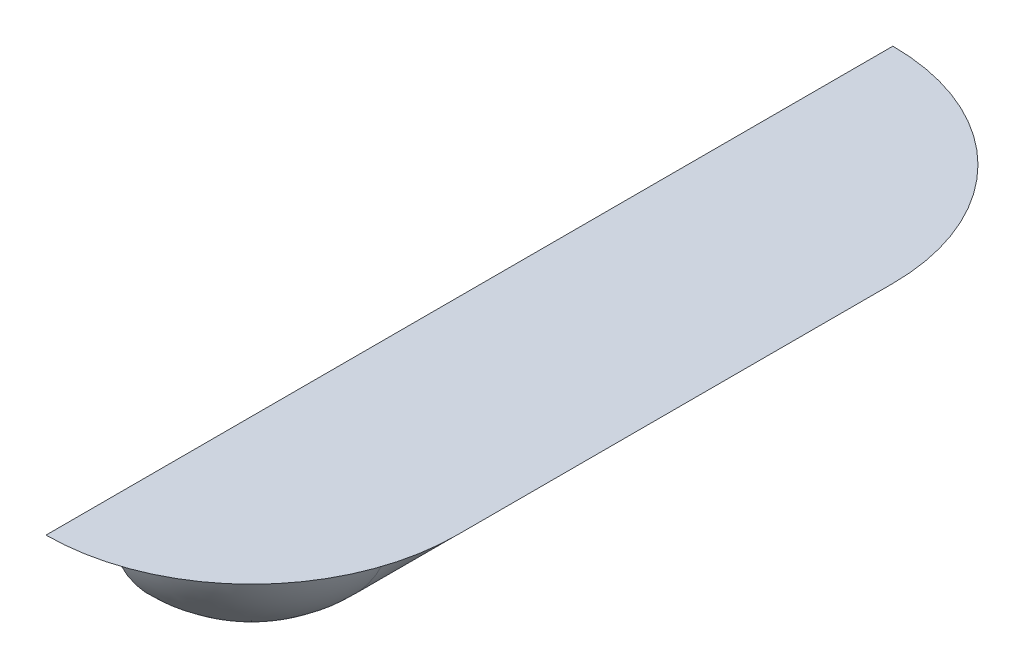
SolidWorks part; units mm, degrees
material "Plain Carbon Steel"
ref_plane "Plane1" through (0, 0, 0) normal (0, 0, 1) x (1, 0, 0)
ref_plane "Plane2" through (0, 0, 0) normal (0, 1, 0) x (1, 0, 0)
ref_plane "Plane3" through (0, 0, 0) normal (1, 0, 0) x (0, 0, -1)
sketch "Base Profile Sketch" plane through (0, 0, 0) normal (0, 0, 1) x (1, 0, 0)
  line L0 (-25, 0) -> (25, 0)
  line L1 (-25, 0) -> (-25, 3.4642)
  line L2 (25, 3.4642) -> (-25, 3.4642)
  line L3 (25, 3.4642) -> (25, 0)
  line L4 (0, 0) -> (0, 3.4642) construction
  line L5 (50, 0) -> (-50, 0) construction
  dimension "D1" = 50
  dimension "D2" = 3.4642
extrude "Base Extrusion 150" add sketch "Base Profile Sketch" along normal mid plane 150
sketch "Layout Sketch" plane through (0, 0, 0) normal (0, -1, 0) x (1, 0, 0)
  line L0 (-6.5173, 0) -> (7.2244, 0) construction
  line L1 (11.2638, 0) -> (-11.2638, 0) construction
  line L2 (0, 9.1132) -> (0, -7.6236) construction
  line L3 (0, -50) -> (0, 50) construction
  line L9 (-10, -50) -> (-10, 50)
  line L11 (10, 30) -> (10, -30)
  arc A0 (10, 30) -> (-10, 50) centre (-10, 30) ccw
  arc A1 (10, -30) -> (-10, -50) centre (-10, -30) cw
  dimension "Overall width" = 100
  dimension "Depth" = 20
sketch "Louver Body" plane through (0, 0, 0) normal (0, 0, 1) x (1, 0, 0)
  line L0 (-10, 0) -> (-10, -20)
  line L1 (-25, 0) -> (25, 0) construction
  line L2 (-10, 0) -> (10, 0)
  line L4 (10, 0) -> (10, 3.4642) construction
  line L5 (25, 3.4642) -> (-25, 3.4642) construction
  line L6 (-10, -20) -> (-3.0249, -20) construction
  line L8 (0, 3.4642) -> (0, 0) construction
  arc A0 (-10, -20) -> (10, 0) centre (-10, 0) ccw
extrude "Louver Boss" add sketch "Louver Body" along normal mid plane 60
sketch "Upper Curl Profile" plane through (0, 0, 30) normal (0, 0, 1) x (1, 0, 0)
  line L0 (-10, 0) -> (-10, -20) construction
  line L1 (-10, 0) -> (-10, -20) construction
  line L2 (-25, 0) -> (25, 0) construction
  line L5 (10, 0) -> (-10, 0)
  line L6 (-10, 0) -> (-10, -20)
  line L7 (10, 0) -> (-10, 0)
  line L8 (-10, 0) -> (-10, -20)
  arc A0 (-10, -20) -> (10, 0) centre (-10, 0) ccw construction
  arc A2 (-10, -20) -> (10, 0) centre (-10, 0) ccw
  arc A3 (-10, -20) -> (10, 0) centre (-10, 0) ccw
  dimension "D1" = 0
revolve "Upper Curl Revolve 90deg" add sketch "Upper Curl Profile" angle 90 about L1
sketch "Lower Curl Profile" plane through (0, 0, -30) normal (0, 0, -1) x (-1, 0, 0)
  line L0 (10, -20) -> (10, 0) construction
  line L1 (25, 0) -> (-25, 0) construction
  line L2 (10, 0) -> (-10, 0)
  line L3 (10, -20) -> (10, 0)
  line L4 (10, 0) -> (-10, 0)
  line L5 (10, -20) -> (10, 0)
  arc A1 (-10, 0) -> (10, -20) centre (10, 0) ccw
  arc A2 (-10, 0) -> (10, -20) centre (10, 0) ccw
  dimension "D1" = 0
revolve "Lower Curl Revolve 90deg" add sketch "Lower Curl Profile" angle 90 about L0
fillet "Bottom Fillet R10" radius 10 3 edges at (10, 0, 0) (4.1421, 0, 44.1421) (4.1421, 0, -44.1421)
sketch "Trim Cut Profile" plane through (-25, 0, 0) normal (-1, 0, 0) x (0, 0, 1)
  line L4 (-75, 0) -> (75, 0)
  line L5 (75, 0) -> (75, 3.4642)
  line L6 (75, 3.4642) -> (-75, 3.4642)
  line L7 (-75, 3.4642) -> (-75, 0)
  line L8 (-75, 0) -> (75, 0)
  line L9 (75, 0) -> (75, 3.4642)
  line L10 (75, 3.4642) -> (-75, 3.4642)
  line L11 (-75, 3.4642) -> (-75, 0)
  dimension "D1" = 0
extrude "Louver Trim Cut" cut sketch "Trim Cut Profile" against normal through all
equation "\"Width@Louver Boss\"=\"Overall width@Layout Sketch\"-2*\"Depth@Layout Sketch\""
